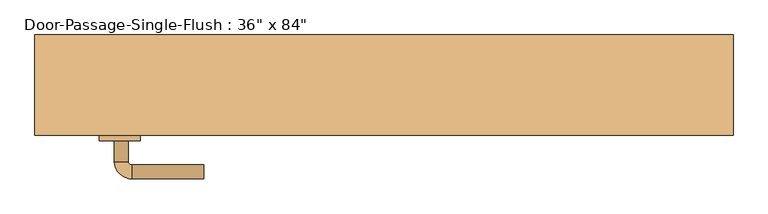
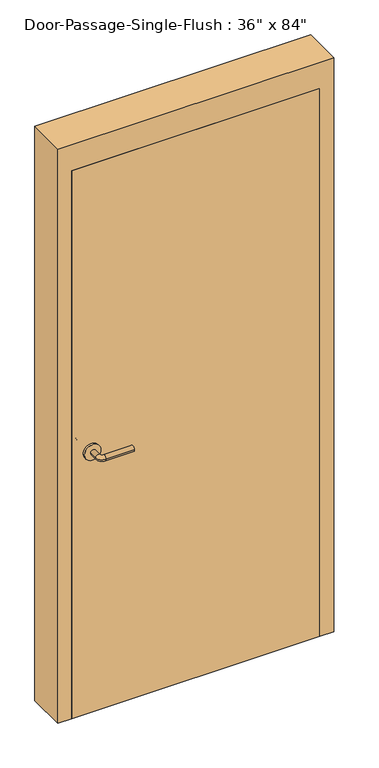
"""IFC4 building model written with IfcOpenShell, lengths in millimetres: door geometry."""

from ifc_helpers import new_model, si_unit, point, frame, frame_2d, origin, origin_with_axes, place, context, project, spatial, polyline, circle_curve, ellipse_curve, trimmed, segment, composite_curve, outline, extrude, faceted_brep, source, transform, mapped, element, save
from ifc_brep_helpers import plane_surface, cylinder_surface, revolved_surface, advanced_brep


def door_9a5ad36a(model_context):
    return source(origin(), model_context, "Body", "SolidModel", [
        advanced_brep(
        [(-392.190625, -42.8, 1016.0), (-372.190625, -42.8, 1016.0), (-392.190625, -12.8, 1016.0), (-372.190625, -12.8, 1016.0), (-367.190625, -7.8, 1016.0), (-367.190625, 12.2, 1016.0), (-262.190625, 12.2, 1016.0), (-262.190625, -7.8, 1016.0)],
        [
            (0, 1, circle_curve(frame((-382.190625, -42.8, 1016.0), z_axis=(0.0, -1.0, 0.0), x_axis=(1.0, 0.0, 0.0)), 10.0)),
            (1, 0, circle_curve(frame((-382.190625, -42.8, 1016.0), z_axis=(0.0, -1.0, 0.0), x_axis=(1.0, 0.0, 0.0)), 10.0)),
            (0, 2),
            (2, 3, circle_curve(frame((-382.190625, -12.8, 1016.0), z_axis=(0.0, -1.0, 0.0), x_axis=(1.0, 0.0, 0.0)), 10.0)),
            (3, 1),
            (3, 2, circle_curve(frame((-382.190625, -12.8, 1016.0), z_axis=(0.0, -1.0, 0.0), x_axis=(1.0, 0.0, 0.0)), 10.0)),
            (4, 3, circle_curve(frame((-367.190625, -12.8, 1016.0), z_axis=(0.0, 0.0, 1.0), x_axis=(-1.0, 0.0, 0.0)), 5.0)),
            (2, 5, circle_curve(frame((-367.190625, -12.8, 1016.0), z_axis=(0.0, 0.0, -1.0), x_axis=(-1.0, 0.0, 0.0)), 25.0)),
            (5, 4, circle_curve(frame((-367.190625, 2.2, 1016.0), z_axis=(-1.0, 0.0, 0.0), x_axis=(0.0, -1.0, 0.0)), 10.0)),
            (4, 5, circle_curve(frame((-367.190625, 2.2, 1016.0), z_axis=(-1.0, 0.0, 0.0), x_axis=(0.0, -1.0, 0.0)), 10.0)),
            (6, 7, circle_curve(frame((-262.190625, 2.2, 1016.0), z_axis=(1.0, 0.0, 0.0), x_axis=(0.0, -1.0, 0.0)), 10.0)),
            (7, 6, circle_curve(frame((-262.190625, 2.2, 1016.0), z_axis=(1.0, 0.0, 0.0), x_axis=(0.0, -1.0, 0.0)), 10.0)),
            (5, 6),
            (7, 4),
        ],
        [
            plane_surface(frame((-382.190625, -42.8, 1016.0), z_axis=(0.0, -1.0, 0.0), x_axis=(0.0, 0.0, 1.0))),
            cylinder_surface(frame((-382.190625, -42.8, 1016.0), z_axis=(0.0, -1.0, 0.0), x_axis=(1.0, 0.0, 0.0)), 10.0),
            revolved_surface(trimmed(ellipse_curve(frame((-382.190625, -12.8, 1016.0), z_axis=(0.0, -1.0, 0.0), x_axis=(1.0, 0.0, 0.0)), 10.0, 10.0), [point((-392.190625, -12.8, 1016.0))], [point((-372.190625, -12.8, 1016.0))], True, "CARTESIAN"), (-367.190625, -12.8, 1016.0), (0.0, 0.0, -1.0)),
            revolved_surface(trimmed(ellipse_curve(frame((-382.190625, -12.8, 1016.0), z_axis=(0.0, -1.0, 0.0), x_axis=(1.0, 0.0, 0.0)), 10.0, 10.0), [point((-372.190625, -12.8, 1016.0))], [point((-392.190625, -12.8, 1016.0))], True, "CARTESIAN"), (-367.190625, -12.8, 1016.0), (0.0, 0.0, -1.0)),
            plane_surface(frame((-262.190625, 2.2, 1016.0), z_axis=(1.0, 0.0, 0.0), x_axis=(0.0, 0.0, 1.0))),
            cylinder_surface(frame((-367.190625, 2.2, 1016.0), z_axis=(-1.0, 0.0, 0.0), x_axis=(0.0, -1.0, 0.0)), 10.0),
        ],
        [
            (0, [[1, 2]]),
            (1, [[-1, 3, 4, 5]]),
            (1, [[-2, -5, 6, -3]]),
            (2, [[7, -4, 8, 9]]),
            (3, [[-8, -6, -7, 10]]),
            (4, [[11, 12]]),
            (5, [[-9, 13, -12, 14]]),
            (5, [[-10, -14, -11, -13]]),
        ],
    ),
        extrude(outline(composite_curve([segment(trimmed(circle_curve(frame_2d((1016.0, -384.690625)), 30.0), [point((1016.0, -414.690625))], [point((1016.0, -354.690625))], False, "CARTESIAN"), True, "CONTINUOUS"), segment(trimmed(circle_curve(frame_2d((1016.0, -384.690625)), 30.0), [point((1016.0, -354.690625))], [point((1016.0, -414.690625))], False, "CARTESIAN"), True, "CONTINUOUS")], self_intersect=False)), frame((0.0, -50.8, 0.0), z_axis=(0.0, 1.0, 0.0), x_axis=(0.0, 0.0, 1.0)), (0.0, 0.0, 1.0), 8.0),
        advanced_brep(
        [(-392.190625, -103.25, 1016.0), (-372.190625, -103.25, 1016.0), (-372.190625, -133.25, 1016.0), (-392.190625, -133.25, 1016.0), (-367.190625, -138.25, 1016.0), (-367.190625, -158.25, 1016.0), (-262.190625, -158.25, 1016.0), (-262.190625, -138.25, 1016.0)],
        [
            (0, 1, circle_curve(frame((-382.190625, -103.25, 1016.0), z_axis=(0.0, 1.0, 0.0), x_axis=(1.0, 0.0, 0.0)), 10.0)),
            (1, 0, circle_curve(frame((-382.190625, -103.25, 1016.0), z_axis=(0.0, 1.0, 0.0), x_axis=(1.0, 0.0, 0.0)), 10.0)),
            (1, 2),
            (2, 3, circle_curve(frame((-382.190625, -133.25, 1016.0), z_axis=(0.0, 1.0, 0.0), x_axis=(1.0, 0.0, 0.0)), 10.0)),
            (3, 0),
            (3, 2, circle_curve(frame((-382.190625, -133.25, 1016.0), z_axis=(0.0, 1.0, 0.0), x_axis=(1.0, 0.0, 0.0)), 10.0)),
            (4, 5, circle_curve(frame((-367.190625, -148.25, 1016.0), z_axis=(-1.0, 0.0, 0.0), x_axis=(0.0, 1.0, 0.0)), 10.0)),
            (5, 3, circle_curve(frame((-367.190625, -133.25, 1016.0), z_axis=(0.0, 0.0, -1.0), x_axis=(-1.0, 0.0, 0.0)), 25.0)),
            (2, 4, circle_curve(frame((-367.190625, -133.25, 1016.0), z_axis=(0.0, 0.0, 1.0), x_axis=(-1.0, 0.0, 0.0)), 5.0)),
            (5, 4, circle_curve(frame((-367.190625, -148.25, 1016.0), z_axis=(-1.0, 0.0, 0.0), x_axis=(0.0, 1.0, 0.0)), 10.0)),
            (6, 7, circle_curve(frame((-262.190625, -148.25, 1016.0), z_axis=(1.0, 0.0, 0.0), x_axis=(0.0, 1.0, 0.0)), 10.0)),
            (7, 6, circle_curve(frame((-262.190625, -148.25, 1016.0), z_axis=(1.0, 0.0, 0.0), x_axis=(0.0, 1.0, 0.0)), 10.0)),
            (4, 7),
            (6, 5),
        ],
        [
            plane_surface(frame((-382.190625, -103.25, 1016.0), z_axis=(0.0, 1.0, 0.0), x_axis=(0.0, 0.0, 1.0))),
            cylinder_surface(frame((-382.190625, -103.25, 1016.0), z_axis=(0.0, 1.0, 0.0), x_axis=(1.0, 0.0, 0.0)), 10.0),
            revolved_surface(trimmed(ellipse_curve(frame((-382.190625, -133.25, 1016.0), z_axis=(0.0, -1.0, 0.0), x_axis=(1.0, 0.0, 0.0)), 10.0, 10.0), [point((-392.190625, -133.25, 1016.0))], [point((-372.190625, -133.25, 1016.0))], True, "CARTESIAN"), (-367.190625, -133.25, 1016.0), (0.0, 0.0, -1.0)),
            revolved_surface(trimmed(ellipse_curve(frame((-382.190625, -133.25, 1016.0), z_axis=(0.0, -1.0, 0.0), x_axis=(1.0, 0.0, 0.0)), 10.0, 10.0), [point((-372.190625, -133.25, 1016.0))], [point((-392.190625, -133.25, 1016.0))], True, "CARTESIAN"), (-367.190625, -133.25, 1016.0), (0.0, 0.0, -1.0)),
            plane_surface(frame((-262.190625, -148.25, 1016.0), z_axis=(1.0, 0.0, 0.0), x_axis=(0.0, 0.0, 1.0))),
            cylinder_surface(frame((-367.190625, -148.25, 1016.0), z_axis=(-1.0, 0.0, 0.0), x_axis=(0.0, 1.0, 0.0)), 10.0),
        ],
        [
            (0, [[1, 2]]),
            (1, [[3, 4, 5, -2]]),
            (1, [[-5, 6, -3, -1]]),
            (2, [[7, 8, -4, 9]]),
            (3, [[10, -9, -6, -8]]),
            (4, [[11, 12]]),
            (5, [[13, -11, 14, -7]]),
            (5, [[-14, -12, -13, -10]]),
        ],
    ),
        extrude(outline(composite_curve([segment(trimmed(circle_curve(frame_2d((1016.0, -384.690625)), 30.0), [point((1016.0, -414.690625))], [point((1016.0, -354.690625))], False, "CARTESIAN"), True, "CONTINUOUS"), segment(trimmed(circle_curve(frame_2d((1016.0, -384.690625)), 30.0), [point((1016.0, -354.690625))], [point((1016.0, -414.690625))], False, "CARTESIAN"), True, "CONTINUOUS")], self_intersect=False)), frame((0.0, -103.25, 0.0), z_axis=(0.0, 1.0, 0.0), x_axis=(0.0, 0.0, 1.0)), (0.0, 0.0, 1.0), 8.0),
        faceted_brep([(457.2, -46.0375, 0.0), (441.325, -46.0375, 0.0), (441.325, 1.5875, 0.0), (457.2, 1.5875, 0.0), (457.2, 50.8, 0.0), (508.0, 50.8, 0.0), (508.0, -95.25, 0.0), (457.2, -95.25, 0.0), (457.2, -95.25, 2133.6), (457.2, -46.0375, 2133.6), (508.0, -95.25, 2235.2), (-508.0, -95.25, 2235.2), (-508.0, -95.25, 0.0), (-457.2, -95.25, 0.0), (-457.2, -95.25, 2133.6), (508.0, 50.8, 2235.2), (457.2, 50.8, 2133.6), (-457.2, 50.8, 2133.6), (-457.2, 50.8, 0.0), (-508.0, 50.8, 0.0), (-508.0, 50.8, 2235.2), (457.2, 1.5875, 2133.6), (441.325, 1.5875, 2117.725), (-441.325, 1.5875, 2117.725), (-441.325, 1.5875, 0.0), (-457.2, 1.5875, 0.0), (-457.2, 1.5875, 2133.6), (441.325, -46.0375, 2117.725), (-457.2, -46.0375, 2133.6), (-457.2, -46.0375, 0.0), (-441.325, -46.0375, 0.0), (-441.325, -46.0375, 2117.725)], [[[0, 1, 2, 3, 4, 5, 6, 7]], [[7, 8, 9, 0]], [[6, 10, 11, 12, 13, 14, 8, 7]], [[5, 15, 10, 6]], [[4, 16, 17, 18, 19, 20, 15, 5]], [[3, 21, 16, 4]], [[2, 22, 23, 24, 25, 26, 21, 3]], [[1, 27, 22, 2]], [[0, 9, 28, 29, 30, 31, 27, 1]], [[8, 14, 28, 9]], [[16, 21, 26, 17]], [[22, 27, 31, 23]], [[12, 19, 18, 25, 24, 30, 29, 13]], [[13, 29, 28, 14]], [[11, 20, 19, 12]], [[17, 26, 25, 18]], [[23, 31, 30, 24]], [[15, 20, 11, 10]]]),
        extrude(outline(polyline([(457.2, -50.8), (457.2, -95.25), (-457.2, -95.25), (-457.2, -50.8), (457.2, -50.8)])), origin_with_axes(), (0.0, 0.0, 1.0), 2133.6),
    ])


if __name__ == "__main__":
    model = new_model("IFC4")
    model_context = context("Model", 3, world=origin())
    ifc_project = project(units=[si_unit("LENGTHUNIT", "METRE", prefix="MILLI")], contexts=[model_context])
    site = spatial("IfcSite", under=ifc_project)
    building = spatial("IfcBuilding", under=site)
    placement = place(None, origin())
    door_shape = door_9a5ad36a(model_context)
    element("IfcDoor", 1, ObjectType="Door-Passage-Single-Flush : 36\" x 84\"", at=placement, inside=building, context=model_context, shape_type="MappedRepresentation", body=[
        mapped(door_shape, transform((0.0, 0.0, 0.0), x_axis=(1.0, 0.0, 0.0), y_axis=(0.0, 1.0, 0.0), z_axis=(0.0, 0.0, 1.0))),
    ])
    save(model, "model.ifc")

# Revit data of these elements
# Type "Door-Passage-Single-Flush : 36\" x 84\""
#   Type Mark = "11"
#   Assembly Code = "B2030200"
#   Analytic Construction = "Wooden"
#   Thickness = 0' - 1 3/4"
#   Thermal Resistance (R) = 2.5876 (h·ft²·°F)/BTU
#   Swing Angle [instance default] = 90.00°
#   Strike Height = 3' - 4"
#   Rough Width [instance default] = 3' - 4"
#   Rough Height [instance default] = 7' - 4"
#   MF Opening Height [instance default] = 0' - 4"
#   MF Opening Width [instance default] = 0' - 4"
#   Inset Calculate [instance default] = 0' - 4"
#   Masonry Inset [instance default] = 0' - 1"
#   Height = 7' - 0"
#   Width = 3' - 0"
#   Heat Transfer Coefficient (U) = 0.3865 BTU/(h·ft²·°F)
#   Masonry Frame Depth = 0' - 5 3/4"
#   Masonry Frame [instance default] = yes
#   Function = 1
#   Dry Wall Frame [instance default] = no
#   Define Thermal Properties by = 1
#   Panel Material = Wood - Birch
#   Frame Material = Metal - Paint Finish - Grey
#   Door Handle Material = Aluminum
#   Visual Light Transmittance = 0
#   Solar Heat Gain Coefficient = 0
#   Wall Closure = (empty or 0)
# Element 1 (IfcDoor, "Door-Passage-Single-Flush : 36\" x 84\"")
#   Materials on its faces: "Aluminum", "Metal - Paint Finish - Grey", "Wood - Birch"
# Materials
#   "Wood - Birch": class "Wood", colour RGB 173 132 96, transparency 0, Cost = 0
#   "Metal - Paint Finish - Grey": class "Paint", colour RGB 178 178 178, transparency 0, Cost = 0
#   "Aluminum": class "Metal", colour RGB 244 245 246, transparency 0, Description = "Aluminum 6061", Cost = 0
